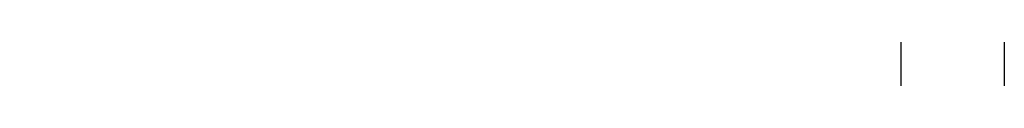
# Model space of a CAD drawing. Units: inches. Extents: x 2091 to 2899, y 967 to 2217.
# Tile 34 of 256: x 2390 to 2459, y 1089 to 1091. Entities that reach past the tile are written whole.
import ezdxf

# ---------------------------------------------------------------- set-up
doc = ezdxf.new("R2010")
doc.units = ezdxf.units.IN
doc.layers.add('A-ANNO-DIMS', color=2, linetype='Continuous', lineweight=18)
doc.styles.get("Standard").update_dxf_attribs({"font": 'arial.ttf'})
doc.dimstyles.new('ISO-25', dxfattribs={"dimtxt": 4, "dimasz": 4, "dimexe": 1.25, "dimexo": 0.625, "dimtad": 1, "dimdec": 0, "dimlunit": 3, "dimtxsty": 'Standard', "dimcen": 2.5, "dimadec": 0, "dimazin": 0, "dimtfac": 1, "dimtdec": 0, "dimtmove": 0, "dimatfit": 3, "dimfxl": 1, "dimarcsym": 0})

# ---------------------------------------------------------------- blocks, each defined once
blk = doc.blocks.new('*D68')
at = {"layer": 'A-ANNO-DIMS', "color": 0, "lineweight": -2, "transparency": 16777216}
for p, q in [((2317.144, 1535.794), (2317.144, 969.464)), ((2459.384, 1535.794), (2459.384, 969.464)), ((2321.144, 970.714), (2455.384, 970.714))]:
    blk.add_line(p, q, dxfattribs=at)
at = {"layer": 'A-ANNO-DIMS', "color": 0, "transparency": 16777216}
for points in [[(2321.144, 971.381), (2321.144, 970.048), (2317.144, 970.714)], [(2455.384, 971.381), (2455.384, 970.048), (2459.384, 970.714)]]:
    blk.add_solid(points, dxfattribs=at)
at = {"layer": 'Defpoints', "color": 0, "transparency": 16777216}
for p in [(2317.144, 1536.419), (2459.384, 1536.419), (2459.384, 970.714)]:
    blk.add_point(p, dxfattribs=at)
at = {"layer": 'A-ANNO-DIMS', "color": 0, "transparency": 16777216, "insert": (2388.264, 973.382), "char_height": 4, "attachment_point": 5}
blk.add_mtext('11\'-10"', dxfattribs=at)
blk = doc.blocks.new('*D71')
at = {"layer": 'A-ANNO-DIMS', "color": 0, "lineweight": -2, "transparency": 16777216}
for p, q in [((2212.144, 1351.294), (2212.144, 969.464)), ((2452.144, 1351.294), (2452.144, 969.464)), ((2216.144, 970.714), (2448.144, 970.714))]:
    blk.add_line(p, q, dxfattribs=at)
at = {"layer": 'A-ANNO-DIMS', "color": 0, "transparency": 16777216}
for points in [[(2216.144, 971.381), (2216.144, 970.048), (2212.144, 970.714)], [(2448.144, 971.381), (2448.144, 970.048), (2452.144, 970.714)]]:
    blk.add_solid(points, dxfattribs=at)
at = {"layer": 'Defpoints', "color": 0, "transparency": 16777216}
for p in [(2212.144, 1351.919), (2452.144, 1351.919), (2452.144, 970.714)]:
    blk.add_point(p, dxfattribs=at)
at = {"layer": 'A-ANNO-DIMS', "color": 0, "transparency": 16777216, "insert": (2332.144, 973.382), "char_height": 4, "attachment_point": 5}
blk.add_mtext('20\'-0"', dxfattribs=at)

msp = doc.modelspace()

# ---------------------------------------------------------------- dimensions: what is measured, and where the dimension line sits
at = {"layer": 'A-ANNO-DIMS'}
for base, p1, p2, picture, middle in [((2459.384, 970.714), (2317.144, 1536.419), (2459.384, 1536.419), '*D68', (2388.264, 973.382)), ((2452.144, 970.714), (2212.144, 1351.919), (2452.144, 1351.919), '*D71', (2332.144, 973.382))]:
    dim = msp.add_linear_dim(base=base, p1=p1, p2=p2, dimstyle='ISO-25', override={"dimdec": 1, "dimlfac": 1, "dimrnd": 0, "dimzin": 1, "dimdsep": 46, "dimlunit": 4, "dimfrac": 2}, dxfattribs=at)
    dim.commit()
    dim.dimension.update_dxf_attribs({"geometry": picture, "text_midpoint": middle})

doc.saveas('drawing.dxf')
